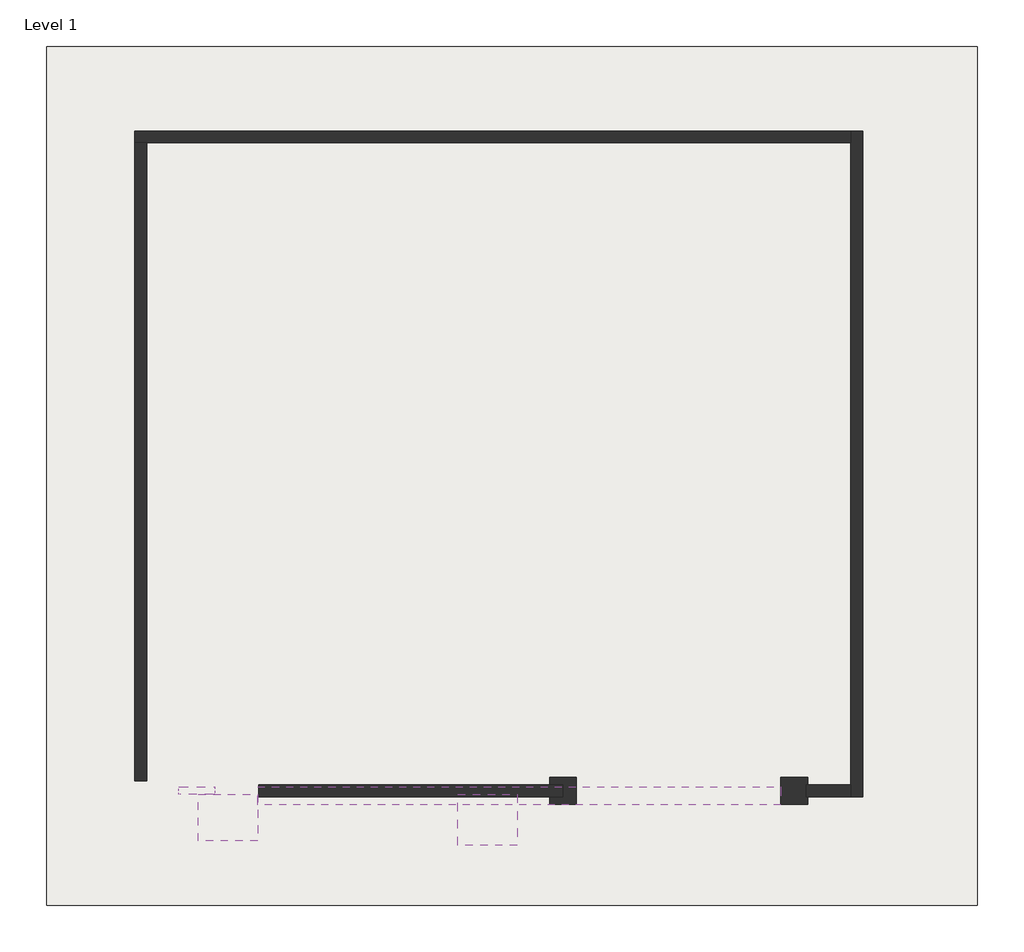
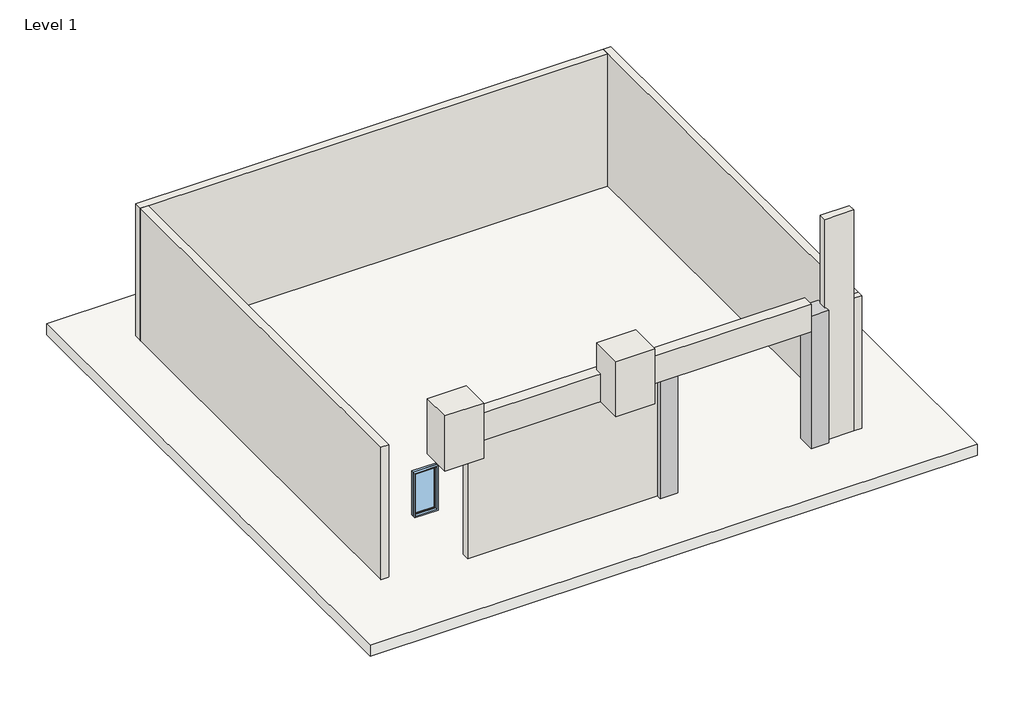
# One storey: 8 walls, 2 columns, 1 slab, 1 window.
"""IFC4 building model written with IfcOpenShell, lengths in millimetres."""

from ifc_helpers import new_model, si_unit, frame, origin, origin_with_axes, place, context, project, spatial, polyline, outline, extrude, faceted_brep, transform, mapped, element, save
from components import walls_1_walls_1_d9e15aa8, walls_2_walls_2_1c393272, walls_3_walls_1_4af12cd7, window_4879aceb

model = new_model("IFC4")

# Units and contexts
model_context = context("Model", 3, world=origin())
ifc_project = project(units=[si_unit("LENGTHUNIT", "METRE", prefix="MILLI")], contexts=[model_context])

# Site, building, storey
site = spatial("IfcSite", under=ifc_project)
building = spatial("IfcBuilding", under=site)
storey = spatial("IfcBuildingStorey", under=building, Name="Level 1", Elevation=0.0)

# Columns
placement = place(None, origin())
element("IfcColumn", 1, ObjectType="Rectangular Column : 18\" x 18\"", at=placement, inside=storey, context=model_context, shape_type="Brep", body=[
    faceted_brep([(-8247.130251, 3042.773096, 3657.6), (-8704.330251, 3042.773096, 3657.6), (-8704.330251, 2585.573096, 3657.6), (-8247.130251, 2585.573096, 3657.6), (-8247.130251, 3042.773096, 0.0), (-8247.130251, 2585.573096, 0.0), (-8704.330251, 2585.573096, 0.0), (-8704.330251, 2712.573096, 0.0), (-8475.730251, 2712.573096, 0.0), (-8475.730251, 2915.773096, 0.0), (-8704.330251, 2915.773096, 0.0), (-8704.330251, 3042.773096, 0.0), (-8704.330251, 2915.773096, 3239.9410058), (-8704.330251, 2712.573096, 3239.9410058), (-8475.730251, 2712.573096, 3239.9410058), (-8475.730251, 2915.773096, 3239.9410058)], [[[0, 1, 2, 3]], [[4, 5, 6, 7, 8, 9, 10, 11]], [[1, 0, 4, 11]], [[2, 1, 11, 10, 12, 13, 7, 6]], [[3, 2, 6, 5]], [[0, 3, 5, 4]], [[14, 8, 7, 13]], [[9, 15, 12, 10]], [[8, 14, 15, 9]], [[15, 14, 13, 12]]]),
])
element("IfcColumn", 2, ObjectType="Rectangular Column : 18\" x 18\"", at=placement, inside=storey, context=model_context, shape_type="SweptSolid", body=[
    extrude(outline(polyline([(-4310.130251, 2585.573096), (-4767.330251, 2585.573096), (-4767.330251, 3042.773096), (-4310.130251, 3042.773096), (-4310.130251, 2915.773096), (-4335.530251, 2915.773096), (-4335.530251, 2712.573096), (-4310.130251, 2712.573096), (-4310.130251, 2585.573096)])), origin_with_axes(), (0.0, 0.0, 1.0), 3657.6),
])

# Slab
element("IfcSlab", 3, ObjectType="Generic - 12\"", at=placement, inside=storey, context=model_context, shape_type="SweptSolid", body=[
    extrude(outline(polyline([(-1418.8612913, 15492.4228948), (-1418.8612913, 862.0228948), (-17268.4612913, 862.0228948), (-17268.4612913, 15492.4228948), (-1418.8612913, 15492.4228948)])), frame((0.0, 0.0, -304.8), z_axis=(0.0, 0.0, 1.0), x_axis=(1.0, 0.0, 0.0)), (0.0, 0.0, 1.0), 304.8),
])

# Walls
element("IfcWall", 4, ObjectType="Generic - 8\"", at=placement, inside=storey, context=model_context, shape_type="Brep", body=[
    faceted_brep([(-15765.530251, 13850.473096, 0.0), (-15562.330251, 13850.473096, 0.0), (-3573.530251, 13850.473096, 0.0), (-3573.530251, 13850.473096, 3657.6), (-15562.330251, 13850.473096, 3657.6), (-15765.530251, 13850.473096, 3657.6), (-15765.530251, 14053.673096, 0.0), (-15765.530251, 14053.673096, 3657.6), (-3573.530251, 14053.673096, 3657.6), (-3573.530251, 14053.673096, 0.0)], [[[0, 1, 2, 3, 4, 5]], [[6, 7, 8, 9]], [[2, 1, 0, 6, 9]], [[0, 5, 7, 6]], [[3, 2, 9, 8]], [[5, 4, 3, 8, 7]]]),
])
element("IfcWall", 5, ObjectType="Generic - 8\"", at=placement, inside=storey, context=model_context, shape_type="SweptSolid", body=[
    extrude(outline(polyline([(-15562.330251, 13850.473096), (-15562.330251, 2979.273096), (-15765.530251, 2979.273096), (-15765.530251, 13850.473096), (-15562.330251, 13850.473096)])), origin_with_axes(), (0.0, 0.0, 1.0), 3657.6),
])
element("IfcWall", 6, ObjectType="Generic - 8\"", at=placement, inside=storey, context=model_context, shape_type="Brep", body=[
    faceted_brep([(-3573.530251, 14053.673096, 0.0), (-3573.530251, 13850.473096, 0.0), (-3573.530251, 2915.773096, 0.0), (-3573.530251, 2712.573096, 0.0), (-3573.530251, 2712.573096, 3657.6), (-3573.530251, 2877.673096, 3657.6), (-3573.530251, 13850.473096, 3657.6), (-3573.530251, 14053.673096, 3657.6), (-3370.330251, 14053.673096, 0.0), (-3370.330251, 14053.673096, 3657.6), (-3370.330251, 2877.673096, 3657.6), (-3370.330251, 2712.573096, 3657.6), (-3370.330251, 2712.573096, 0.0)], [[[0, 1, 2, 3, 4, 5, 6, 7]], [[8, 9, 10, 11, 12]], [[3, 2, 1, 0, 8, 12]], [[0, 7, 9, 8]], [[5, 4, 11, 10]], [[7, 6, 5, 10, 9]], [[4, 3, 12, 11]]]),
])
element("IfcWall", 7, ObjectType="Generic - 8\"", at=placement, inside=storey, context=model_context, shape_type="Brep", body=[
    faceted_brep([(-13657.330251, 2712.573096, 0.0), (-8704.330251, 2712.573096, 0.0), (-8475.730251, 2712.573096, 0.0), (-8475.730251, 2712.573096, 3239.9410058), (-8704.330251, 2712.573096, 3239.9410058), (-13657.330251, 2712.573096, 3239.9410058), (-13657.330251, 2915.773096, 0.0), (-13657.330251, 2915.773096, 3239.9410058), (-8704.330251, 2915.773096, 3239.9410058), (-8475.730251, 2915.773096, 3239.9410058), (-8475.730251, 2915.773096, 0.0), (-8704.330251, 2915.773096, 0.0), (-13657.330251, 2750.673096, 0.0), (-13657.330251, 2877.673096, 0.0)], [[[0, 1, 2, 3, 4, 5]], [[6, 7, 8, 9, 10, 11]], [[2, 1, 0, 12, 13, 6, 11, 10]], [[3, 2, 10, 9]], [[5, 4, 3, 9, 8, 7]], [[0, 5, 7, 6, 13, 12]]]),
])
element("IfcWall", 8, ObjectType="Generic - 8\"", at=placement, inside=storey, context=model_context, shape_type="Brep", body=[
    faceted_brep([(-3573.530251, 2915.773096, 0.0), (-4310.130251, 2915.773096, 0.0), (-4335.530251, 2915.773096, 0.0), (-4335.530251, 2915.773096, 3657.6), (-4335.530251, 2915.773096, 6096.0), (-3573.530251, 2915.773096, 6096.0), (-3573.530251, 2712.573096, 0.0), (-3573.530251, 2712.573096, 3657.6), (-3573.530251, 2712.573096, 6096.0), (-4335.530251, 2712.573096, 6096.0), (-4335.530251, 2712.573096, 3657.6), (-4335.530251, 2712.573096, 0.0), (-4310.130251, 2712.573096, 0.0)], [[[0, 1, 2, 3, 4, 5]], [[6, 7, 8, 9, 10, 11, 12]], [[2, 1, 0, 6, 12, 11]], [[4, 3, 2, 11, 10, 9]], [[5, 4, 9, 8]], [[0, 5, 8, 7, 6]]]),
])
walls_1_walls_1_shape = walls_1_walls_1_d9e15aa8(model_context)
element("IfcWall", 9, ObjectType="Walls 1 : Walls 1", at=placement, inside=storey, context=model_context, shape_type="MappedRepresentation", body=[
    mapped(walls_1_walls_1_shape, transform((0.0, 0.0, 0.0), x_axis=(1.0, 0.0, 0.0), y_axis=(0.0, 1.0, 0.0), z_axis=(0.0, 0.0, 1.0))),
])
walls_2_walls_2_shape = walls_2_walls_2_1c393272(model_context)
element("IfcWall", 10, ObjectType="Walls 2 : Walls 2", at=placement, inside=storey, context=model_context, shape_type="MappedRepresentation", body=[
    mapped(walls_2_walls_2_shape, transform((0.0, 0.0, 0.0), x_axis=(1.0, 0.0, 0.0), y_axis=(0.0, 1.0, 0.0), z_axis=(0.0, 0.0, 1.0))),
])
walls_3_walls_1_shape = walls_3_walls_1_4af12cd7(model_context)
element("IfcWall", 11, ObjectType="Walls 3 : Walls 1", at=placement, inside=storey, context=model_context, shape_type="MappedRepresentation", body=[
    mapped(walls_3_walls_1_shape, transform((4419.6, 0.0, -3657.6), x_axis=(1.0, 0.0, 0.0), y_axis=(0.0, 1.0, 0.0), z_axis=(0.0, 0.0, 1.0))),
])

# Window
window_shape = window_4879aceb(model_context)
element("IfcWindow", 12, ObjectType="Fixed : 24\" x 48\"", at=placement, inside=storey, context=model_context, shape_type="MappedRepresentation", body=[
    mapped(window_shape, transform((-14673.330251, 2814.173096, 672.8056944), x_axis=(1.0, 0.0, 0.0), y_axis=(0.0, 1.0, 0.0), z_axis=(0.0, 0.0, 1.0))),
])

save(model, "model.ifc")

# Revit data of these elements
# Type "Rectangular Column : 18\" x 18\""
#   Assembly Code = "B1010200"
#   Depth = 1' - 6"
#   Offset Base = 0' - 0"
#   Offset Top = 0' - 0"
#   Width = 1' - 6"
#   Material = none
# Type "Generic - 12\""
#   Assembly Code = "B1010"
#   Function = 0
#   Layers, outside or top first: 1' - 0" no material (function 1)
# Type "Generic - 8\""
#   Assembly Code = "B2010"
#   Layers, outside or top first: 0' - 8" no material (function 1)
# Type "Fixed : 24\" x 48\""
#   Type Mark = "2"
#   Construction Type Id = "GSP4R"
#   Assembly Code = "B2020100"
#   Analytic Construction = "1/8 in Pilkington single glazing"
#   Visual Light Transmittance = 0.9
#   Solar Heat Gain Coefficient = 0.78
#   Heat Transfer Coefficient (U) = 0.6496 BTU/(h·ft²·°F)
#   Height = 4' - 0"
#   Default Sill Height = 3' - 0"
#   Width = 2' - 0"
#   Window Inset = 0' - 0 3/4"
#   Define Thermal Properties by = 1
#   Glass Pane Material = Glass
#   Sash Material = Sash
#   Wall Closure = (empty or 0)
# Elements 1, 2 (IfcColumn, "Rectangular Column : 18\" x 18\"")
#   Phase Created = New Construction
#   Materials on its faces: "Default Wall"
# Element 3 (IfcSlab, "Generic - 12\"")
#   Height Offset From Level = 0' - 0"
#   Phase Created = New Construction
#   Materials on its faces: "Default Floor"
# Elements 4, 5, 6 (IfcWall, "Generic - 8\"")
#   Top Offset = 0' - 0"
#   Base Offset = 0' - 0"
#   Unconnected Height = 12' - 0"
#   wall height = 12' - 0"
#   Phase Created = New Construction
#   Base Constraint = Level 1
#   Materials on its faces: "Default Wall"
# Element 7 (IfcWall, "Generic - 8\"")
#   Top Offset = 0' - 0"
#   Base Offset = 0' - 0"
#   Unconnected Height = 10' - 7.55673"
#   wall height = 10' - 7.55673"
#   Phase Created = New Construction
#   Base Constraint = Level 1
#   Materials on its faces: "Default Wall"
# Element 8 (IfcWall, "Generic - 8\"")
#   Top Offset = 0' - 0"
#   Base Offset = 0' - 0"
#   Unconnected Height = 20' - 0"
#   wall height = 20' - 0"
#   Phase Created = New Construction
#   Base Constraint = Level 1
#   Materials on its faces: "Default Wall"
# Element 9 (IfcWall, "Walls 1 : Walls 1")
#   Phase Created = New Construction
#   Materials on its faces: "Default Wall"
# Element 10 (IfcWall, "Walls 2 : Walls 2")
#   Phase Created = New Construction
#   Materials on its faces: "Default Wall"
# Element 11 (IfcWall, "Walls 3 : Walls 1")
#   Phase Created = New Construction
#   Materials on its faces: "Default Wall"
# Element 12 (IfcWindow, "Fixed : 24\" x 48\"")
#   Mark = "7"
#   Phase Created = New Construction
#   Materials on its faces: "Sash", "Glass"
# Materials
#   "Glass": class "Glass", colour RGB 0 128 192, transparency 0.75, Description = "Soda Lime Glass", Cost = 0
#   "Sash": class "Wood", colour RGB 224 178 126, transparency 0
#   "Default Wall": colour RGB 128 128 128, transparency 0
#   "Default Floor": colour RGB 128 128 128, transparency 0
